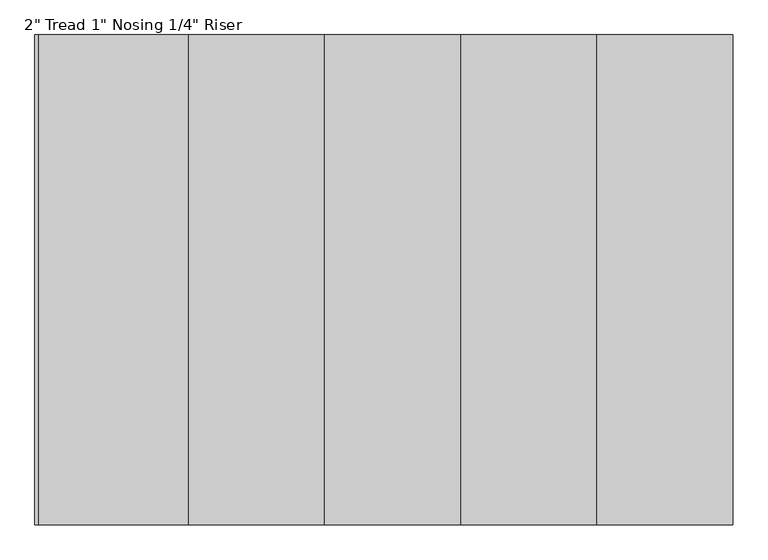
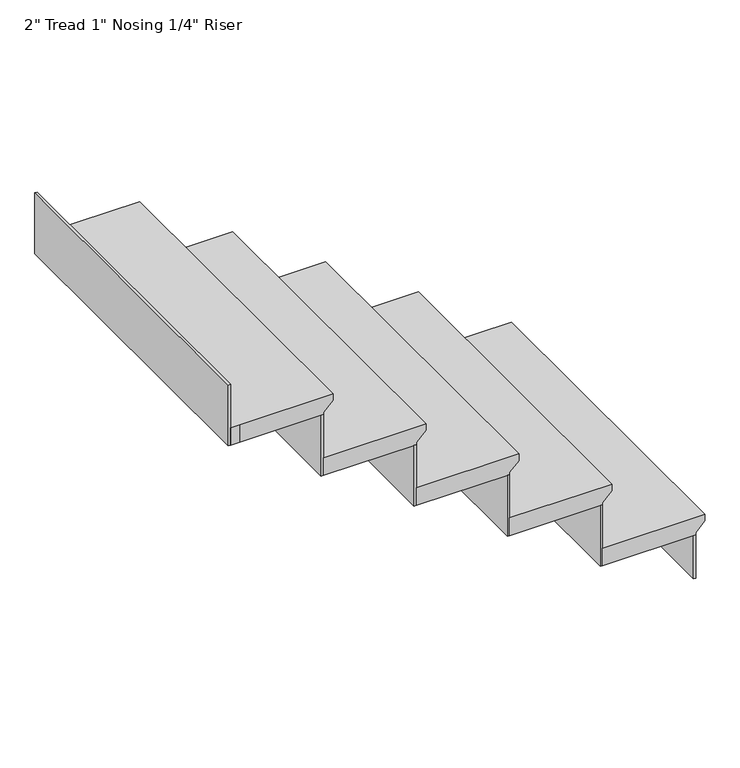
"""IFC4 building model written with IfcOpenShell, lengths in millimetres: stair flight geometry."""

from ifc_helpers import new_model, si_unit, origin, place, context, project, spatial, faceted_brep, source, transform, mapped, element, save


def stair_flight_0f448409(model_context):
    return source(origin(), model_context, "Body", "Brep", [
        faceted_brep([(-3329.9669727, -4867.8688563, 156.7961538), (-3329.9669727, -4867.8688563, 175.8461538), (-3329.9669727, -5782.2688563, 175.8461538), (-3329.9669727, -5782.2688563, 156.7961538), (-3355.3669727, -4867.8688563, 131.3961538), (-3355.3669727, -5782.2688563, 131.3961538), (-3609.3669727, -4867.8688563, 175.8461538), (-3609.3669727, -5782.2688563, 175.8461538), (-3355.3669727, -5782.2688563, 125.0461538), (-3609.3669727, -5782.2688563, 125.0461538), (-3609.3669727, -4867.8688563, 125.0461538), (-3355.3669727, -4867.8688563, 125.0461538)], [[[0, 1, 2, 3]], [[4, 0, 3, 5]], [[2, 1, 6, 7]], [[8, 9, 10, 11]], [[2, 7, 9, 8, 5, 3]], [[8, 11, 4, 5]], [[6, 1, 0, 4, 11, 10]], [[7, 6, 10, 9]]]),
        faceted_brep([(-3355.3669727, -4867.8688563, 125.0461538), (-3355.3669727, -4867.8688563, 0.0), (-3361.7169727, -4867.8688563, 0.0), (-3361.7169727, -4867.8688563, 125.0461538), (-3355.3669727, -5782.2688563, 125.0461538), (-3361.7169727, -5782.2688563, 125.0461538), (-3361.7169727, -5782.2688563, 0.0), (-3355.3669727, -5782.2688563, 0.0)], [[[0, 1, 2, 3]], [[4, 5, 6, 7]], [[1, 0, 4, 7]], [[2, 1, 7, 6]], [[3, 2, 6, 5]], [[0, 3, 5, 4]]]),
        faceted_brep([(-3609.3669727, -4867.8688563, 300.8923077), (-3609.3669727, -4867.8688563, 125.0461538), (-3615.7169727, -4867.8688563, 125.0461538), (-3615.7169727, -4867.8688563, 300.8923077), (-3609.3669727, -5782.2688563, 300.8923077), (-3615.7169727, -5782.2688563, 300.8923077), (-3615.7169727, -5782.2688563, 125.0461538), (-3609.3669727, -5782.2688563, 125.0461538)], [[[0, 1, 2, 3]], [[4, 5, 6, 7]], [[1, 0, 4, 7]], [[2, 1, 7, 6]], [[3, 2, 6, 5]], [[0, 3, 5, 4]]]),
        faceted_brep([(-3583.9669727, -5782.2688563, 351.6923077), (-3583.9669727, -4867.8688563, 351.6923077), (-3863.3669727, -4867.8688563, 351.6923077), (-3863.3669727, -5782.2688563, 351.6923077), (-3609.3669727, -5782.2688563, 300.8923077), (-3863.3669727, -5782.2688563, 300.8923077), (-3863.3669727, -4867.8688563, 300.8923077), (-3609.3669727, -4867.8688563, 300.8923077), (-3609.3669727, -5782.2688563, 307.2423077), (-3583.9669727, -5782.2688563, 332.6423077), (-3609.3669727, -4867.8688563, 307.2423077), (-3583.9669727, -4867.8688563, 332.6423077)], [[[0, 1, 2, 3]], [[4, 5, 6, 7]], [[0, 3, 5, 4, 8, 9]], [[4, 7, 10, 8]], [[2, 1, 11, 10, 7, 6]], [[3, 2, 6, 5]], [[11, 1, 0, 9]], [[10, 11, 9, 8]]]),
        faceted_brep([(-3863.3669727, -4867.8688563, 476.7384615), (-3863.3669727, -4867.8688563, 300.8923077), (-3869.7169727, -4867.8688563, 300.8923077), (-3869.7169727, -4867.8688563, 476.7384615), (-3863.3669727, -5782.2688563, 476.7384615), (-3869.7169727, -5782.2688563, 476.7384615), (-3869.7169727, -5782.2688563, 300.8923077), (-3863.3669727, -5782.2688563, 300.8923077)], [[[0, 1, 2, 3]], [[4, 5, 6, 7]], [[1, 0, 4, 7]], [[2, 1, 7, 6]], [[3, 2, 6, 5]], [[0, 3, 5, 4]]]),
        faceted_brep([(-3837.9669727, -5782.2688563, 527.5384615), (-3837.9669727, -4867.8688563, 527.5384615), (-4117.3669727, -4867.8688563, 527.5384615), (-4117.3669727, -5782.2688563, 527.5384615), (-3863.3669727, -5782.2688563, 476.7384615), (-4117.3669727, -5782.2688563, 476.7384615), (-4117.3669727, -4867.8688563, 476.7384615), (-3863.3669727, -4867.8688563, 476.7384615), (-3863.3669727, -5782.2688563, 483.0884615), (-3837.9669727, -5782.2688563, 508.4884615), (-3863.3669727, -4867.8688563, 483.0884615), (-3837.9669727, -4867.8688563, 508.4884615)], [[[0, 1, 2, 3]], [[4, 5, 6, 7]], [[0, 3, 5, 4, 8, 9]], [[4, 7, 10, 8]], [[2, 1, 11, 10, 7, 6]], [[3, 2, 6, 5]], [[11, 1, 0, 9]], [[10, 11, 9, 8]]]),
        faceted_brep([(-4117.3669727, -4867.8688563, 652.5846154), (-4117.3669727, -4867.8688563, 476.7384615), (-4123.7169727, -4867.8688563, 476.7384615), (-4123.7169727, -4867.8688563, 652.5846154), (-4117.3669727, -5782.2688563, 652.5846154), (-4123.7169727, -5782.2688563, 652.5846154), (-4123.7169727, -5782.2688563, 476.7384615), (-4117.3669727, -5782.2688563, 476.7384615)], [[[0, 1, 2, 3]], [[4, 5, 6, 7]], [[1, 0, 4, 7]], [[2, 1, 7, 6]], [[3, 2, 6, 5]], [[0, 3, 5, 4]]]),
        faceted_brep([(-4091.9669727, -5782.2688563, 703.3846154), (-4091.9669727, -4867.8688563, 703.3846154), (-4371.3669727, -4867.8688563, 703.3846154), (-4371.3669727, -5782.2688563, 703.3846154), (-4117.3669727, -5782.2688563, 652.5846154), (-4371.3669727, -5782.2688563, 652.5846154), (-4371.3669727, -4867.8688563, 652.5846154), (-4117.3669727, -4867.8688563, 652.5846154), (-4117.3669727, -5782.2688563, 658.9346154), (-4091.9669727, -5782.2688563, 684.3346154), (-4117.3669727, -4867.8688563, 658.9346154), (-4091.9669727, -4867.8688563, 684.3346154)], [[[0, 1, 2, 3]], [[4, 5, 6, 7]], [[0, 3, 5, 4, 8, 9]], [[4, 7, 10, 8]], [[2, 1, 11, 10, 7, 6]], [[3, 2, 6, 5]], [[11, 1, 0, 9]], [[10, 11, 9, 8]]]),
        faceted_brep([(-4625.3669727, -4867.8688563, 1004.2769231), (-4625.3669727, -4867.8688563, 828.4307692), (-4631.7169727, -4867.8688563, 828.4307692), (-4631.7169727, -4867.8688563, 1004.2769231), (-4625.3669727, -5782.2688563, 1004.2769231), (-4631.7169727, -5782.2688563, 1004.2769231), (-4631.7169727, -5782.2688563, 828.4307692), (-4625.3669727, -5782.2688563, 828.4307692)], [[[0, 1, 2, 3]], [[4, 5, 6, 7]], [[1, 0, 4, 7]], [[2, 1, 7, 6]], [[3, 2, 6, 5]], [[0, 3, 5, 4]]]),
        faceted_brep([(-4371.3669727, -4867.8688563, 828.4307692), (-4371.3669727, -4867.8688563, 652.5846154), (-4377.7169727, -4867.8688563, 652.5846154), (-4377.7169727, -4867.8688563, 828.4307692), (-4371.3669727, -5782.2688563, 828.4307692), (-4377.7169727, -5782.2688563, 828.4307692), (-4377.7169727, -5782.2688563, 652.5846154), (-4371.3669727, -5782.2688563, 652.5846154)], [[[0, 1, 2, 3]], [[4, 5, 6, 7]], [[1, 0, 4, 7]], [[2, 1, 7, 6]], [[3, 2, 6, 5]], [[0, 3, 5, 4]]]),
        faceted_brep([(-4625.3669727, -5782.2688563, 879.2307692), (-4599.9669727, -5782.2688563, 879.2307692), (-4345.9669727, -5782.2688563, 879.2307692), (-4345.9669727, -4867.8688563, 879.2307692), (-4599.9669727, -4867.8688563, 879.2307692), (-4625.3669727, -4867.8688563, 879.2307692), (-4599.9669727, -5782.2688563, 828.4307692), (-4625.3669727, -5782.2688563, 828.4307692), (-4625.3669727, -4867.8688563, 828.4307692), (-4599.9669727, -4867.8688563, 828.4307692), (-4371.3669727, -4867.8688563, 828.4307692), (-4371.3669727, -5782.2688563, 828.4307692), (-4371.3669727, -5782.2688563, 834.7807692), (-4345.9669727, -5782.2688563, 860.1807692), (-4371.3669727, -4867.8688563, 834.7807692), (-4345.9669727, -4867.8688563, 860.1807692)], [[[0, 1, 2, 3, 4, 5]], [[6, 7, 8, 9, 10, 11]], [[1, 0, 7, 6]], [[2, 1, 6, 11, 12, 13]], [[11, 10, 14, 12]], [[4, 3, 15, 14, 10, 9]], [[5, 4, 9, 8]], [[0, 5, 8, 7]], [[15, 3, 2, 13]], [[14, 15, 13, 12]]]),
    ])


if __name__ == "__main__":
    model = new_model("IFC4")
    model_context = context("Model", 3, world=origin())
    ifc_project = project(units=[si_unit("LENGTHUNIT", "METRE", prefix="MILLI")], contexts=[model_context])
    site = spatial("IfcSite", under=ifc_project)
    building = spatial("IfcBuilding", under=site)
    placement = place(None, origin())
    stair_flight_shape = stair_flight_0f448409(model_context)
    element("IfcStairFlight", 1, ObjectType="2\" Tread 1\" Nosing 1/4\" Riser", at=placement, inside=building, context=model_context, shape_type="MappedRepresentation", body=[
        mapped(stair_flight_shape, transform((0.0, 0.0, 0.0), x_axis=(1.0, 0.0, 0.0), y_axis=(0.0, 1.0, 0.0), z_axis=(0.0, 0.0, 1.0))),
    ])
    save(model, "model.ifc")
